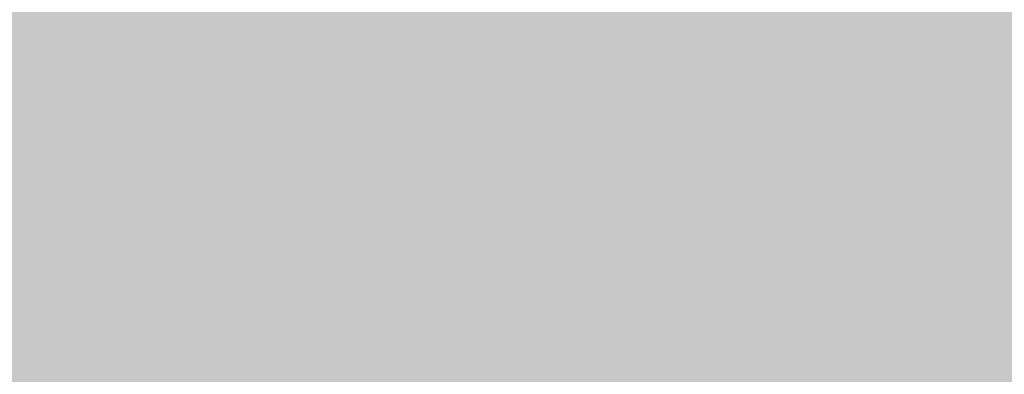
# Model space of a CAD drawing. Units: feet. Extents: x 3168 to 4724, y 827 to 1477.
# Tile 183 of 256: x 3307.378 to 3316.072, y 1093.654 to 1096.781. Entities that reach past the tile are written whole.
import ezdxf

# ---------------------------------------------------------------- set-up
doc = ezdxf.new("R2010")
doc.units = ezdxf.units.FT
doc.layers.add('A-ELEV-PATT', color=8, linetype='Continuous', lineweight=13)

msp = doc.modelspace()

# ---------------------------------------------------------------- hatches: boundary and pattern name
at = {"layer": 'A-ELEV-PATT'}
h = msp.add_hatch(color=256, dxfattribs=at)
h.dxf.hatch_style = 1
edge = h.paths.add_edge_path()
edge.add_ellipse((3552.9058, 979.2201), major_axis=(36.7449, 0), ratio=0.4848485, start_angle=0, end_angle=360)
edge = h.paths.add_edge_path()
edge.add_ellipse((3559.8916, 929.2523), major_axis=(36.7449, 0), ratio=0.4848485, start_angle=0, end_angle=360)
edge = h.paths.add_edge_path()
edge.add_line((3299.3168, 1198.6061), (3479.9167, 1198.6061))
edge.add_line((3479.9167, 1198.6061), (3479.9167, 1209.8686))
edge.add_spline(control_points=[(3479.9167, 1209.8686), (3464.3012, 1209.8686), (3448.6856, 1209.8686), (3410.9491, 1209.8686), (3388.8282, 1209.8686), (3355.6469, 1209.8686), (3344.5864, 1209.8686), (3327.9957, 1209.8686), (3322.4655, 1209.8686), (3314.1702, 1209.8686), (3311.4051, 1209.8686), (3307.2574, 1209.8686), (3305.8748, 1209.8686), (3303.801, 1209.8686), (3303.1097, 1209.8686), (3302.0728, 1209.8686), (3301.7272, 1209.8686), (3301.2087, 1209.8686), (3301.0359, 1209.8686), (3300.7767, 1209.8686), (3300.6903, 1209.8686), (3300.5606, 1209.8686), (3300.5174, 1209.8686), (3300.4526, 1209.8686), (3300.431, 1209.8686), (3300.3986, 1209.8686), (3300.3878, 1209.8686), (3300.3662, 1209.8686), (3300.3457, 1209.8686), (3300.3455, 1209.8686), (3300.3455, 1209.8686), (3300.3433, 1209.8686), (3300.3411, 1209.8686), (3300.3379, 1209.8686), (3300.3368, 1209.8686), (3300.3339, 1209.8686), (3300.3321, 1209.8686), (3300.3255, 1209.8686), (3300.3207, 1209.8686), (3300.3109, 1209.8686), (3300.306, 1209.8686), (3300.2905, 1209.8686), (3300.28, 1209.8686), (3300.2324, 1209.8688), (3300.1953, 1209.869), (3299.9511, 1209.8706), (3299.7448, 1209.8743), (3299.4368, 1209.8833), (3299.3344, 1209.8868), (3299.1811, 1209.8929), (3299.13, 1209.8951), (3298.6522, 1209.9168), (3298.2295, 1209.9457), (3297.6016, 1210.0024), (3297.3934, 1210.0235), (3297.0827, 1210.0583), (3296.9793, 1210.0705), (3296.293, 1210.1549), (3295.7181, 1210.2434), (3294.8687, 1210.3989), (3294.5877, 1210.4545), (3294.1693, 1210.5433), (3294.0304, 1210.5739), (3291.7071, 1211.1012), (3289.6536, 1211.8134), (3285.7763, 1213.564), (3283.9514, 1214.6035), (3280.5122, 1216.9801), (3278.8972, 1218.3176), (3276.3799, 1220.8295), (3275.416, 1221.9177), (3274.0393, 1223.7077), (3273.581, 1224.3495), (3273.1432, 1225.0163)], knot_values=[39.119033, 39.119033, 39.119033, 39.119033, 39.286353, 39.286353, 39.523379, 39.523379, 39.641892, 39.641892, 39.701148, 39.701148, 39.730777, 39.730777, 39.745591, 39.745591, 39.752998, 39.752998, 39.756701, 39.756701, 39.758553, 39.758553, 39.759479, 39.759479, 39.759942, 39.759942, 39.760173, 39.760173, 39.760289, 39.760289, 39.760405, 39.760405, 39.760463, 39.760463, 39.763389, 39.763389, 39.764851, 39.764851, 39.767304, 39.767304, 39.773825, 39.773825, 39.78057, 39.78057, 39.79477, 39.79477, 39.845194, 39.845194, 40.126715, 40.126715, 40.267476, 40.267476, 40.337856, 40.337856, 40.927023, 40.927023, 41.221606, 41.221606, 41.368898, 41.368898, 42.202622, 42.202622, 42.619485, 42.619485, 42.827916, 42.827916, 46.118323, 46.118323, 49.408731, 49.408731, 52.699139, 52.699139, 54.927489, 54.927489, 56.104228, 56.104228, 56.104228, 56.104228], weights=[1, 1, 1, 1, 1, 1, 1, 1, 1, 1, 1, 1, 1, 1, 1, 1, 1, 1, 1, 1, 1, 1, 1, 1, 1, 1, 1, 1, 1, 1, 1, 1, 1, 1, 1, 1, 1, 1, 1, 1, 1, 1, 1, 1, 1, 1, 1, 1, 1, 1, 1, 1, 1, 1, 1, 1, 1, 1, 1, 1, 1, 1, 1, 1, 1, 1, 1, 1, 1, 1, 1, 1, 1, 1], degree=3, periodic=0)
edge.add_line((3273.1432, 1225.0163), (3273.1432, 1099.0163))
edge.add_line((3273.1432, 1099.0163), (3299.3168, 1099.0163))
edge.add_line((3299.3168, 1099.0163), (3299.3168, 1198.6061))
edge = h.paths.add_edge_path()
edge.add_line((3304.7584, 1324.1581), (3479.9167, 1324.1581))
edge.add_line((3479.9167, 1324.1581), (3479.9167, 1335.7146))
edge.add_line((3479.9167, 1335.7146), (3269.1616, 1335.7146))
edge.add_spline(control_points=[(3269.1616, 1335.7146), (3264.0242, 1335.7146), (3258.3641, 1328.9582), (3259.2643, 1323.9003)], knot_values=[0, 0, 0, 0, 15.412191, 15.412191, 15.412191, 15.412191], degree=3, periodic=0)
edge.add_line((3259.2643, 1323.9003), (3265.5168, 1288.7691))
edge.add_line((3265.5168, 1288.7691), (3275.2651, 1261.5456))
edge.add_line((3275.2651, 1261.5456), (3304.7584, 1261.5456))
edge.add_line((3304.7584, 1261.5456), (3304.7584, 1324.1581))
h = msp.add_hatch(color=256, dxfattribs=at)
h.dxf.hatch_style = 1
h.paths.add_polyline_path([(3384.5252, 1099.0163), (3335.0292, 1099.0163), (3299.3168, 1099.0163), (3273.1432, 1099.0163), (3217.5654, 1099.0163), (3168.0693, 827.1163), (3335.0292, 827.1163)])

doc.saveas('drawing.dxf')
